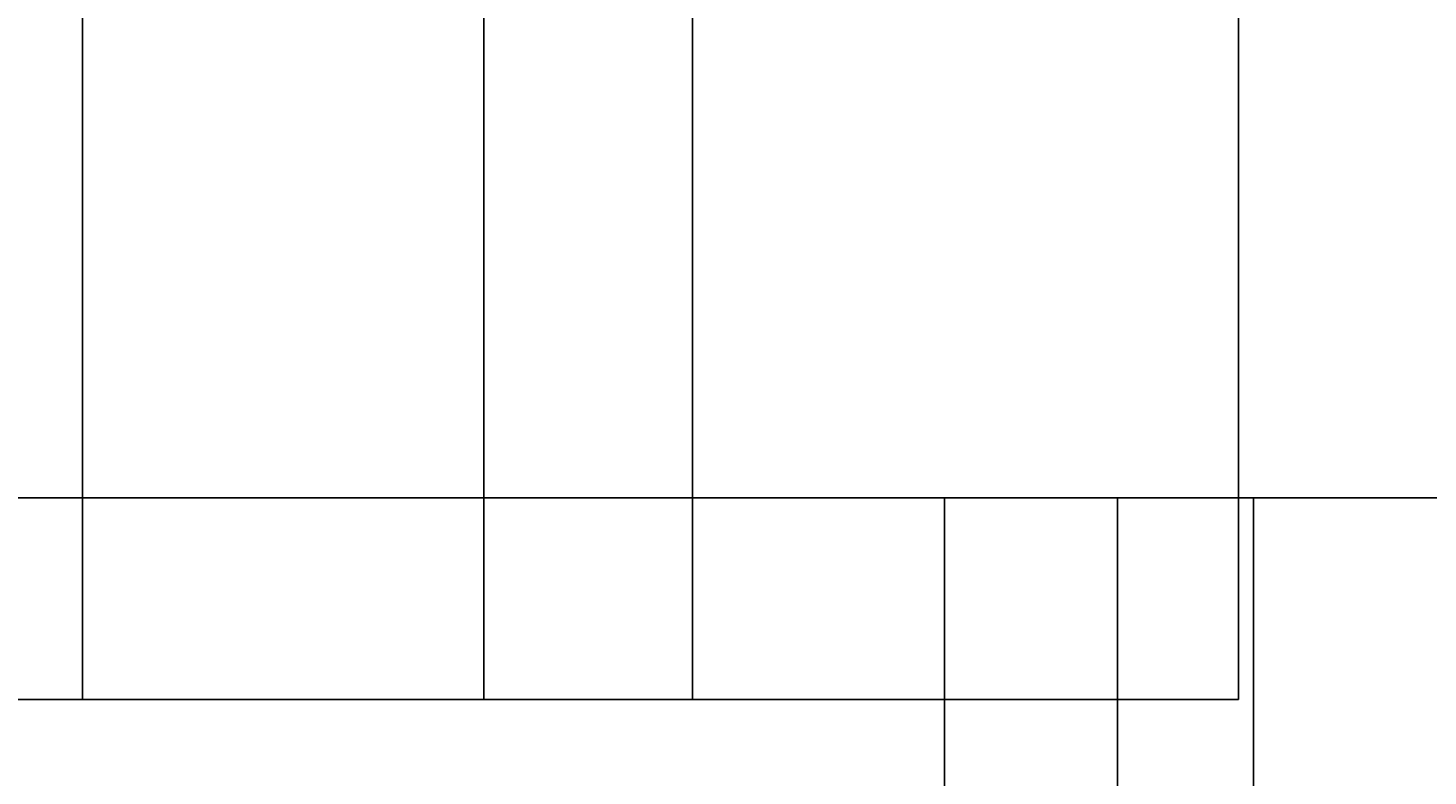
# Model space of a CAD drawing. Units: inches. Extents: x -32109 to 33221, y -19197 to 7608.
# Tile 19 of 25: x 12337 to 19011, y -5795 to -2226. Entities that reach past the tile are written whole.
import ezdxf

# ---------------------------------------------------------------- set-up
doc = ezdxf.new("R2010")
doc.units = ezdxf.units.IN
doc.header["$MEASUREMENT"] = 0
doc.layers.add('A-ANNO-DIMS', color=2, linetype='Continuous', lineweight=18)
doc.styles.get("Standard").update_dxf_attribs({"font": 'arial.ttf'})
doc.dimstyles.get("Standard").update_dxf_attribs({"dimtxt": 0.18, "dimasz": 0.18, "dimexe": 0.18, "dimexo": 0.0625, "dimgap": 0.09, "dimtad": 0, "dimtih": 1, "dimtoh": 1, "dimdec": 4, "dimzin": 0, "dimdsep": 46, "dimtxsty": 'Standard', "dimcen": 0.09, "dimadec": 0, "dimazin": 0, "dimtfac": 1, "dimtdec": 4, "dimtofl": 0, "dimtmove": 0, "dimatfit": 3, "dimfxl": 1, "dimtolj": 1, "dimtzin": 0, "dimarcsym": 0})

# ---------------------------------------------------------------- blocks, each defined once
blk = doc.blocks.new('*D16')
at = {"layer": 'A-ANNO-DIMS', "color": 0, "lineweight": -2, "transparency": 16777216}
for p, q in [((7931.9, -8929), (7931.9, -4467.1)), ((7932, -4467.3), (18774.7, -4467.3)), ((29618.2, -4467.3), (18775.5, -4467.3)), ((29618.3, -6090.7), (29618.3, -4467.1))]:
    blk.add_line(p, q, dxfattribs=at)
at = {"layer": 'A-ANNO-DIMS', "color": 0, "transparency": 16777216}
for points in [[(7932, -4467.2), (7932, -4467.3), (7931.9, -4467.3)], [(29618.2, -4467.2), (29618.2, -4467.3), (29618.3, -4467.3)]]:
    blk.add_solid(points, dxfattribs=at)
at = {"layer": 'Defpoints', "color": 0, "transparency": 16777216}
for p in [(29618.3, -4467.3), (29618.3, -6090.8), (7931.9, -8929.1)]:
    blk.add_point(p, dxfattribs=at)
at = {"layer": 'A-ANNO-DIMS', "color": 0, "transparency": 16777216, "insert": (18775.1, -4467.3), "char_height": 0.18, "attachment_point": 5}
blk.add_mtext('\\A1;21686', dxfattribs=at)
blk = doc.blocks.new('*D19')
at = {"layer": 'A-ANNO-DIMS', "color": 0, "lineweight": -2, "transparency": 16777216}
for p, q in [((16706.7, -6693.3), (16706.7, -4467.1)), ((16706.9, -4467.3), (21231.6, -4467.3)), ((25757.1, -4467.3), (21232.3, -4467.3)), ((25757.3, -6693.3), (25757.3, -4467.1))]:
    blk.add_line(p, q, dxfattribs=at)
at = {"layer": 'A-ANNO-DIMS', "color": 0, "transparency": 16777216}
for points in [[(16706.9, -4467.2), (16706.9, -4467.3), (16706.7, -4467.3)], [(25757.1, -4467.2), (25757.1, -4467.3), (25757.3, -4467.3)]]:
    blk.add_solid(points, dxfattribs=at)
at = {"layer": 'Defpoints', "color": 0, "transparency": 16777216}
for p in [(25757.3, -4467.3), (16706.7, -6693.4), (25757.3, -6693.4)]:
    blk.add_point(p, dxfattribs=at)
at = {"layer": 'A-ANNO-DIMS', "color": 0, "transparency": 16777216, "insert": (21232, -4467.3), "char_height": 0.18, "attachment_point": 5}
blk.add_mtext('\\A1;9051', dxfattribs=at)
blk = doc.blocks.new('*D62')
at = {"layer": 'A-ANNO-DIMS', "color": 0, "lineweight": -2, "transparency": 16777216}
for p, q in [((12596.6, 1705.1), (12596.6, -5429.7)), ((11383.7, -2116.2), (11383.7, -5429.7)), ((11383.9, -5429.6), (11989.8, -5429.6)), ((12596.5, -5429.6), (11990.5, -5429.6))]:
    blk.add_line(p, q, dxfattribs=at)
at = {"layer": 'A-ANNO-DIMS', "color": 0, "transparency": 16777216}
for points in [[(11383.9, -5429.5), (11383.9, -5429.6), (11383.7, -5429.6)], [(12596.5, -5429.5), (12596.5, -5429.6), (12596.6, -5429.6)]]:
    blk.add_solid(points, dxfattribs=at)
at = {"layer": 'Defpoints', "color": 0, "transparency": 16777216}
for p in [(12596.6, 1705.2), (11383.7, -2116.1), (12596.6, -5429.6)]:
    blk.add_point(p, dxfattribs=at)
at = {"layer": 'A-ANNO-DIMS', "color": 0, "transparency": 16777216, "insert": (11990.2, -5429.6), "char_height": 0.18, "attachment_point": 5}
blk.add_mtext('\\A1;1213', dxfattribs=at)
blk = doc.blocks.new('*D63')
at = {"layer": 'A-ANNO-DIMS', "color": 0, "lineweight": -2, "transparency": 16777216}
for p, q in [((12596.6, 1705.1), (12596.6, -5429.7)), ((14509.6, 1705.1), (14509.6, -5429.7)), ((12596.8, -5429.6), (13552.7, -5429.6)), ((14509.4, -5429.6), (13553.4, -5429.6))]:
    blk.add_line(p, q, dxfattribs=at)
at = {"layer": 'A-ANNO-DIMS', "color": 0, "transparency": 16777216}
for points in [[(12596.8, -5429.5), (12596.8, -5429.6), (12596.6, -5429.6)], [(14509.4, -5429.5), (14509.4, -5429.6), (14509.6, -5429.6)]]:
    blk.add_solid(points, dxfattribs=at)
at = {"layer": 'Defpoints', "color": 0, "transparency": 16777216}
for p in [(12596.6, 1705.2), (14509.6, 1705.2), (14509.6, -5429.6)]:
    blk.add_point(p, dxfattribs=at)
at = {"layer": 'A-ANNO-DIMS', "color": 0, "transparency": 16777216, "insert": (13553.1, -5429.6), "char_height": 0.18, "attachment_point": 5}
blk.add_mtext('\\A1;1913', dxfattribs=at)
blk = doc.blocks.new('*D64')
at = {"layer": 'A-ANNO-DIMS', "color": 0, "lineweight": -2, "transparency": 16777216}
for p, q in [((14509.6, 1705.1), (14509.6, -5429.7)), ((15505.7, -101.7), (15505.7, -5429.7)), ((14509.7, -5429.6), (15007.3, -5429.6)), ((15505.6, -5429.6), (15008, -5429.6))]:
    blk.add_line(p, q, dxfattribs=at)
at = {"layer": 'A-ANNO-DIMS', "color": 0, "transparency": 16777216}
for points in [[(14509.7, -5429.5), (14509.7, -5429.6), (14509.6, -5429.6)], [(15505.6, -5429.5), (15505.6, -5429.6), (15505.7, -5429.6)]]:
    blk.add_solid(points, dxfattribs=at)
at = {"layer": 'Defpoints', "color": 0, "transparency": 16777216}
for p in [(14509.6, 1705.2), (15505.7, -101.6), (15505.7, -5429.6)]:
    blk.add_point(p, dxfattribs=at)
at = {"layer": 'A-ANNO-DIMS', "color": 0, "transparency": 16777216, "insert": (15007.6, -5429.6), "char_height": 0.18, "attachment_point": 5}
blk.add_mtext('\\A1;996.2', dxfattribs=at)
blk = doc.blocks.new('*D65')
at = {"layer": 'A-ANNO-DIMS', "color": 0, "lineweight": -2, "transparency": 16777216}
for p, q in [((15505.7, -101.7), (15505.7, -5429.7)), ((18108.4, -2136.1), (18108.4, -5429.7)), ((15505.9, -5429.6), (16806.6, -5429.6)), ((18108.2, -5429.6), (16807.5, -5429.6))]:
    blk.add_line(p, q, dxfattribs=at)
at = {"layer": 'A-ANNO-DIMS', "color": 0, "transparency": 16777216}
for points in [[(15505.9, -5429.5), (15505.9, -5429.6), (15505.7, -5429.6)], [(18108.2, -5429.5), (18108.2, -5429.6), (18108.4, -5429.6)]]:
    blk.add_solid(points, dxfattribs=at)
at = {"layer": 'Defpoints', "color": 0, "transparency": 16777216}
for p in [(15505.7, -101.6), (18108.4, -2136), (18108.4, -5429.6)]:
    blk.add_point(p, dxfattribs=at)
at = {"layer": 'A-ANNO-DIMS', "color": 0, "transparency": 16777216, "insert": (16807.1, -5429.6), "char_height": 0.18, "attachment_point": 5}
blk.add_mtext('\\A1;2602.6', dxfattribs=at)
blk = doc.blocks.new('*D152')
at = {"layer": 'A-ANNO-DIMS', "color": 0, "lineweight": -2, "transparency": 16777216}
for p, q in [((17531.2, -7648.2), (17531.2, -4467.1)), ((17531.3, -4467.3), (17854.5, -4467.3)), ((18178.5, -4467.3), (17855.3, -4467.3)), ((18178.7, -7648.2), (18178.7, -4467.1))]:
    blk.add_line(p, q, dxfattribs=at)
at = {"layer": 'A-ANNO-DIMS', "color": 0, "transparency": 16777216}
for points in [[(17531.3, -4467.2), (17531.3, -4467.3), (17531.2, -4467.3)], [(18178.5, -4467.2), (18178.5, -4467.3), (18178.7, -4467.3)]]:
    blk.add_solid(points, dxfattribs=at)
at = {"layer": 'Defpoints', "color": 0, "transparency": 16777216}
for p in [(18178.7, -4467.3), (17531.2, -7648.3), (18178.7, -7648.3)]:
    blk.add_point(p, dxfattribs=at)
at = {"layer": 'A-ANNO-DIMS', "color": 0, "transparency": 16777216, "insert": (17854.9, -4467.3), "char_height": 0.18, "attachment_point": 5}
blk.add_mtext('\\A1;647.5', dxfattribs=at)

msp = doc.modelspace()

# ---------------------------------------------------------------- dimensions: what is measured, and where the dimension line sits
at = {"layer": 'A-ANNO-DIMS'}
for base, p1, p2, override, picture, middle in [((12596.642, -5429.555), (11383.682, -2116.149), (12596.642, 1705.162), {"dimdec": 0, "dimlfac": 1, "dimrnd": 0, "dimzin": 0, "dimdsep": 46, "dimlunit": 2}, '*D62', (11990.162, -5429.555)), ((14509.55, -5429.555), (12596.642, 1705.162), (14509.55, 1705.162), {"dimdec": 0, "dimlfac": 1, "dimrnd": 0, "dimzin": 0, "dimdsep": 46, "dimlunit": 2}, '*D63', (13553.096, -5429.555)), ((15505.744, -5429.555), (14509.55, 1705.162), (15505.744, -101.6), {"dimdec": 1, "dimlfac": 1, "dimrnd": 0, "dimzin": 0, "dimdsep": 46, "dimlunit": 2}, '*D64', (15007.647, -5429.555)), ((18108.369, -5429.555), (15505.744, -101.6), (18108.369, -2136.004), {"dimdec": 1, "dimlfac": 1, "dimrnd": 0, "dimzin": 0, "dimdsep": 46, "dimlunit": 2}, '*D65', (16807.057, -5429.555)), ((29618.33, -4467.266), (7931.857, -8929.065), (29618.33, -6090.794), {"dimdec": 0, "dimlfac": 1, "dimrnd": 0, "dimzin": 0, "dimdsep": 46, "dimlunit": 2}, '*D16', (18775.094, -4467.266)), ((25757.257, -4467.266), (16706.692, -6693.38), (25757.257, -6693.38), {"dimdec": 0, "dimlfac": 1, "dimrnd": 0, "dimzin": 0, "dimdsep": 46, "dimlunit": 2}, '*D19', (21231.975, -4467.266)), ((18178.681, -4467.266), (17531.159, -7648.26), (18178.681, -7648.26), {"dimdec": 1, "dimlfac": 1, "dimrnd": 0, "dimzin": 0, "dimdsep": 46, "dimlunit": 2}, '*D152', (17854.92, -4467.266))]:
    dim = msp.add_linear_dim(base=base, p1=p1, p2=p2, dimstyle='Standard', override=override, dxfattribs=at)
    dim.commit()
    dim.dimension.update_dxf_attribs({"geometry": picture, "text_midpoint": middle})

doc.saveas('drawing.dxf')
